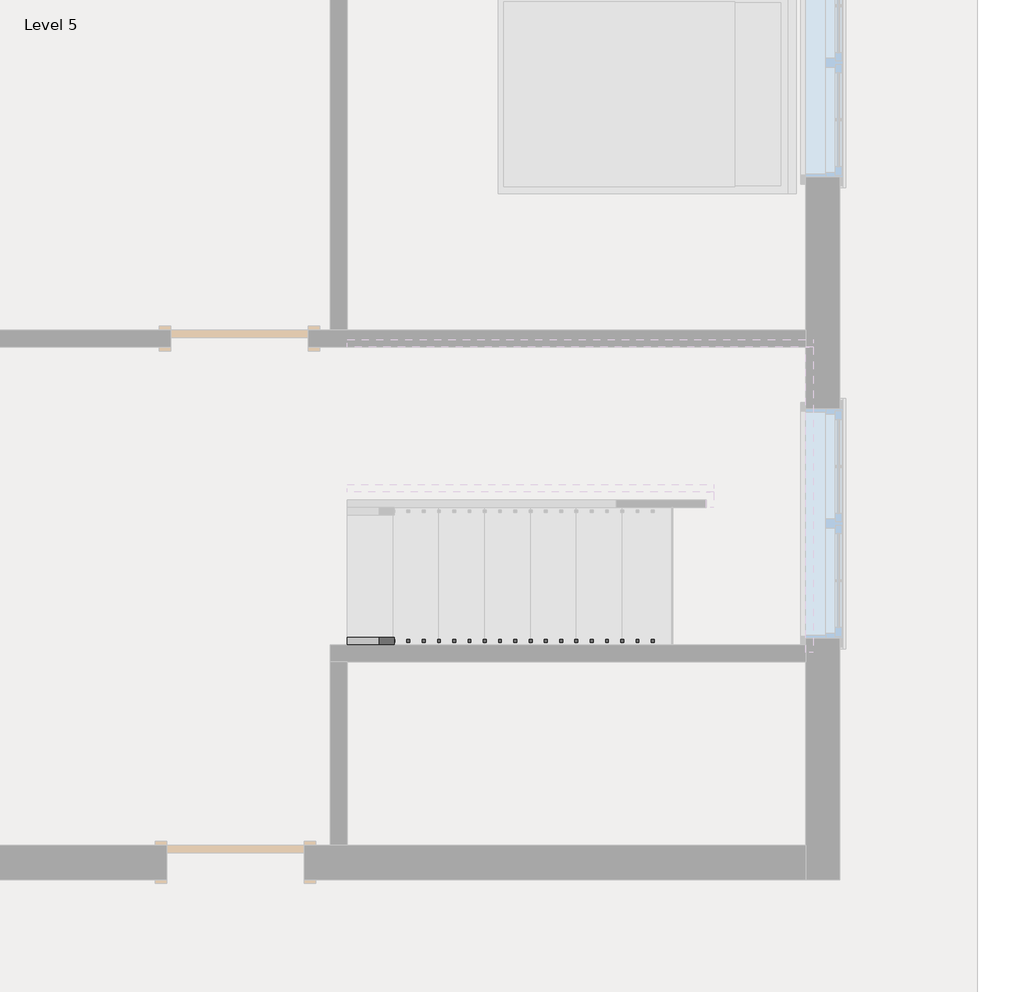
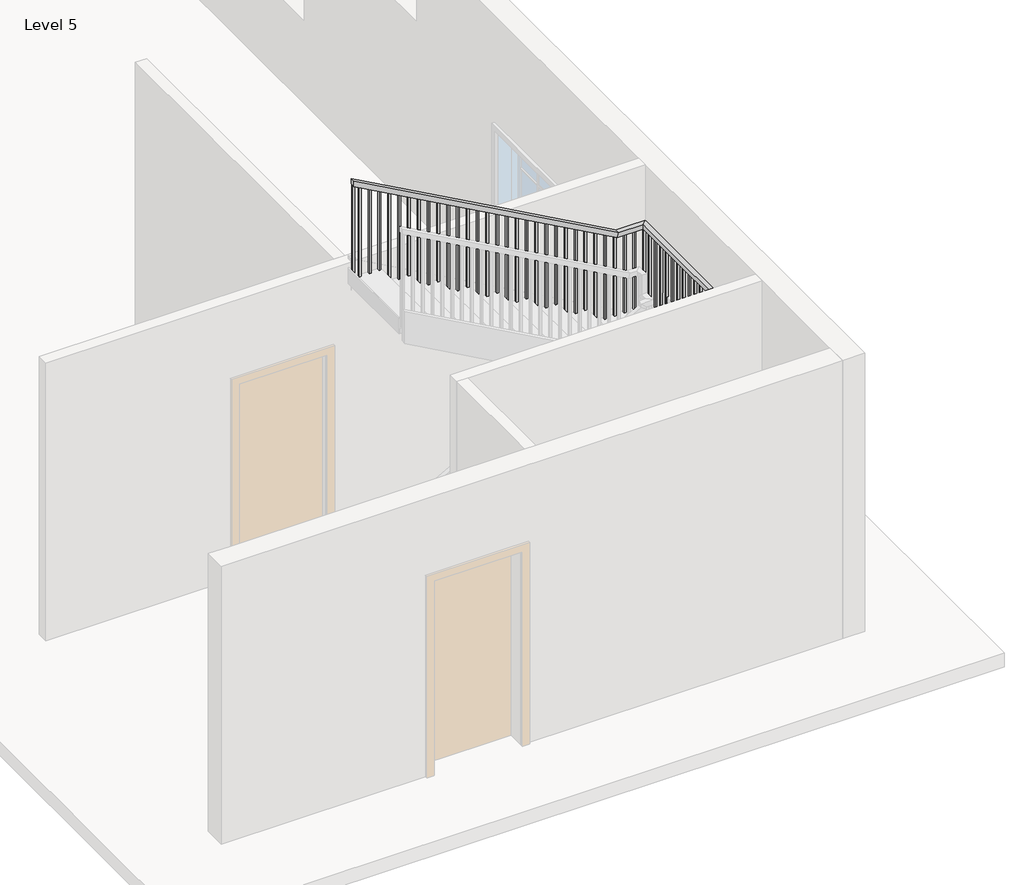
# One storey, part 2 of 3: 1 railing.
"""IFC4 building model written with IfcOpenShell, lengths in millimetres."""

from ifc_helpers import new_model, si_unit, frame, origin, place, context, project, spatial, polyline, outline, extrude, faceted_brep, element, save

model = new_model("IFC4")

# Units and contexts
model_context = context("Model", 3, world=origin())
ifc_project = project(units=[si_unit("LENGTHUNIT", "METRE", prefix="MILLI")], contexts=[model_context])

# Site, building, storey
site = spatial("IfcSite", under=ifc_project)
building = spatial("IfcBuilding", under=site)
storey = spatial("IfcBuildingStorey", under=building, Name="Level 5", Elevation=12649.2)

# Railing
placement = place(None, origin())
element("IfcRailing", 1, ObjectType="Handrail - Rectangular", at=placement, inside=storey, context=model_context, shape_type="SolidModel", body=[
    faceted_brep([(-1197.97188, -4765.70869, 13732.9333333), (-1197.97188, -4765.70869, 13674.820221), (-1197.97188, -4816.50869, 13674.820221), (-1197.97188, -4816.50869, 13732.9333333), (1240.42812, -4765.70869, 15087.6), (1253.5917222, -4765.70869, 15036.8), (1253.5917222, -4816.50869, 15036.8), (1240.42812, -4816.50869, 15087.6), (1799.22812, -4765.70869, 15087.6), (1799.22812, -4765.70869, 15036.8), (1850.02812, -4816.50869, 15036.8), (1850.02812, -4816.50869, 15087.6), (1799.22812, -2886.10869, 15087.6), (1799.22812, -2886.10869, 15036.8), (1850.02812, -2835.30869, 15036.8), (1850.02812, -2835.30869, 15087.6), (1545.22812, -2886.10869, 15087.6), (1532.0645177, -2886.10869, 15036.8), (1532.0645177, -2835.30869, 15036.8), (1545.22812, -2835.30869, 15087.6), (-1197.97188, -2886.10869, 16611.6), (-1197.97188, -2835.30869, 16611.6), (-1197.97188, -2835.30869, 16553.4868876), (-1197.97188, -2886.10869, 16553.4868876)], [[[0, 1, 2, 3]], [[1, 0, 4, 5]], [[2, 1, 5, 6]], [[3, 2, 6, 7]], [[0, 3, 7, 4]], [[5, 4, 8, 9]], [[6, 5, 9, 10]], [[7, 6, 10, 11]], [[4, 7, 11, 8]], [[9, 8, 12, 13]], [[10, 9, 13, 14]], [[11, 10, 14, 15]], [[8, 11, 15, 12]], [[13, 12, 16, 17]], [[14, 13, 17, 18]], [[15, 14, 18, 19]], [[12, 15, 19, 16]], [[20, 21, 22, 23]], [[17, 16, 20, 23]], [[18, 17, 23, 22]], [[19, 18, 22, 21]], [[16, 19, 21, 20]]]),
    extrude(outline(polyline([(16505.8618876, -1112.24688), (16516.445221, -1131.29688), (15527.8666667, -1131.29688), (15527.8666667, -1112.24688), (16505.8618876, -1112.24688)])), frame((0.0, -2870.23369, 0.0), z_axis=(0.0, 1.0, 0.0), x_axis=(0.0, 0.0, 1.0)), (0.0, 0.0, 1.0), 19.05),
    extrude(outline(polyline([(16449.4174432, -1010.64688), (16460.0007765, -1029.69688), (15527.8666667, -1029.69688), (15527.8666667, -1010.64688), (16449.4174432, -1010.64688)])), frame((0.0, -2870.23369, 0.0), z_axis=(0.0, 1.0, 0.0), x_axis=(0.0, 0.0, 1.0)), (0.0, 0.0, 1.0), 19.05),
    extrude(outline(polyline([(16392.9729988, -909.04688), (16403.5563321, -928.09688), (15527.8666667, -928.09688), (15527.8666667, -909.04688), (16392.9729988, -909.04688)])), frame((0.0, -2870.23369, 0.0), z_axis=(0.0, 1.0, 0.0), x_axis=(0.0, 0.0, 1.0)), (0.0, 0.0, 1.0), 19.05),
    extrude(outline(polyline([(16336.5285543, -807.44688), (16347.1118876, -826.49688), (15358.5333333, -826.49688), (15358.5333333, -807.44688), (16336.5285543, -807.44688)])), frame((0.0, -2870.23369, 0.0), z_axis=(0.0, 1.0, 0.0), x_axis=(0.0, 0.0, 1.0)), (0.0, 0.0, 1.0), 19.05),
    extrude(outline(polyline([(16280.0841099, -705.84688), (16290.6674432, -724.89688), (15358.5333333, -724.89688), (15358.5333333, -705.84688), (16280.0841099, -705.84688)])), frame((0.0, -2870.23369, 0.0), z_axis=(0.0, 1.0, 0.0), x_axis=(0.0, 0.0, 1.0)), (0.0, 0.0, 1.0), 19.05),
    extrude(outline(polyline([(16223.6396654, -604.24688), (16234.2229988, -623.29688), (15358.5333333, -623.29688), (15358.5333333, -604.24688), (16223.6396654, -604.24688)])), frame((0.0, -2870.23369, 0.0), z_axis=(0.0, 1.0, 0.0), x_axis=(0.0, 0.0, 1.0)), (0.0, 0.0, 1.0), 19.05),
    extrude(outline(polyline([(16167.195221, -502.64688), (16177.7785543, -521.69688), (15189.2, -521.69688), (15189.2, -502.64688), (16167.195221, -502.64688)])), frame((0.0, -2870.23369, 0.0), z_axis=(0.0, 1.0, 0.0), x_axis=(0.0, 0.0, 1.0)), (0.0, 0.0, 1.0), 19.05),
    extrude(outline(polyline([(16110.7507765, -401.04688), (16121.3341099, -420.09688), (15189.2, -420.09688), (15189.2, -401.04688), (16110.7507765, -401.04688)])), frame((0.0, -2870.23369, 0.0), z_axis=(0.0, 1.0, 0.0), x_axis=(0.0, 0.0, 1.0)), (0.0, 0.0, 1.0), 19.05),
    extrude(outline(polyline([(16054.3063321, -299.44688), (16064.8896654, -318.49688), (15189.2, -318.49688), (15189.2, -299.44688), (16054.3063321, -299.44688)])), frame((0.0, -2870.23369, 0.0), z_axis=(0.0, 1.0, 0.0), x_axis=(0.0, 0.0, 1.0)), (0.0, 0.0, 1.0), 19.05),
    extrude(outline(polyline([(15997.8618876, -197.84688), (16008.445221, -216.89688), (15019.8666667, -216.89688), (15019.8666667, -197.84688), (15997.8618876, -197.84688)])), frame((0.0, -2870.23369, 0.0), z_axis=(0.0, 1.0, 0.0), x_axis=(0.0, 0.0, 1.0)), (0.0, 0.0, 1.0), 19.05),
    extrude(outline(polyline([(15941.4174432, -96.24688), (15952.0007765, -115.29688), (15019.8666667, -115.29688), (15019.8666667, -96.24688), (15941.4174432, -96.24688)])), frame((0.0, -2870.23369, 0.0), z_axis=(0.0, 1.0, 0.0), x_axis=(0.0, 0.0, 1.0)), (0.0, 0.0, 1.0), 19.05),
    extrude(outline(polyline([(15884.9729988, 5.35312), (15895.5563321, -13.69688), (15019.8666667, -13.69688), (15019.8666667, 5.35312), (15884.9729988, 5.35312)])), frame((0.0, -2870.23369, 0.0), z_axis=(0.0, 1.0, 0.0), x_axis=(0.0, 0.0, 1.0)), (0.0, 0.0, 1.0), 19.05),
    extrude(outline(polyline([(15828.5285543, 106.95312), (15839.1118876, 87.90312), (14850.5333333, 87.90312), (14850.5333333, 106.95312), (15828.5285543, 106.95312)])), frame((0.0, -2870.23369, 0.0), z_axis=(0.0, 1.0, 0.0), x_axis=(0.0, 0.0, 1.0)), (0.0, 0.0, 1.0), 19.05),
    extrude(outline(polyline([(15772.0841099, 208.55312), (15782.6674432, 189.50312), (14850.5333333, 189.50312), (14850.5333333, 208.55312), (15772.0841099, 208.55312)])), frame((0.0, -2870.23369, 0.0), z_axis=(0.0, 1.0, 0.0), x_axis=(0.0, 0.0, 1.0)), (0.0, 0.0, 1.0), 19.05),
    extrude(outline(polyline([(15715.6396654, 310.15312), (15726.2229988, 291.10312), (14850.5333333, 291.10312), (14850.5333333, 310.15312), (15715.6396654, 310.15312)])), frame((0.0, -2870.23369, 0.0), z_axis=(0.0, 1.0, 0.0), x_axis=(0.0, 0.0, 1.0)), (0.0, 0.0, 1.0), 19.05),
    extrude(outline(polyline([(15659.195221, 411.75312), (15669.7785543, 392.70312), (14681.2, 392.70312), (14681.2, 411.75312), (15659.195221, 411.75312)])), frame((0.0, -2870.23369, 0.0), z_axis=(0.0, 1.0, 0.0), x_axis=(0.0, 0.0, 1.0)), (0.0, 0.0, 1.0), 19.05),
    extrude(outline(polyline([(15602.7507765, 513.35312), (15613.3341099, 494.30312), (14681.2, 494.30312), (14681.2, 513.35312), (15602.7507765, 513.35312)])), frame((0.0, -2870.23369, 0.0), z_axis=(0.0, 1.0, 0.0), x_axis=(0.0, 0.0, 1.0)), (0.0, 0.0, 1.0), 19.05),
    extrude(outline(polyline([(15546.3063321, 614.95312), (15556.8896654, 595.90312), (14681.2, 595.90312), (14681.2, 614.95312), (15546.3063321, 614.95312)])), frame((0.0, -2870.23369, 0.0), z_axis=(0.0, 1.0, 0.0), x_axis=(0.0, 0.0, 1.0)), (0.0, 0.0, 1.0), 19.05),
    extrude(outline(polyline([(15489.8618876, 716.55312), (15500.445221, 697.50312), (14511.8666667, 697.50312), (14511.8666667, 716.55312), (15489.8618876, 716.55312)])), frame((0.0, -2870.23369, 0.0), z_axis=(0.0, 1.0, 0.0), x_axis=(0.0, 0.0, 1.0)), (0.0, 0.0, 1.0), 19.05),
    extrude(outline(polyline([(15433.4174432, 818.15312), (15444.0007765, 799.10312), (14511.8666667, 799.10312), (14511.8666667, 818.15312), (15433.4174432, 818.15312)])), frame((0.0, -2870.23369, 0.0), z_axis=(0.0, 1.0, 0.0), x_axis=(0.0, 0.0, 1.0)), (0.0, 0.0, 1.0), 19.05),
    extrude(outline(polyline([(15376.9729988, 919.75312), (15387.5563321, 900.70312), (14511.8666667, 900.70312), (14511.8666667, 919.75312), (15376.9729988, 919.75312)])), frame((0.0, -2870.23369, 0.0), z_axis=(0.0, 1.0, 0.0), x_axis=(0.0, 0.0, 1.0)), (0.0, 0.0, 1.0), 19.05),
    extrude(outline(polyline([(15320.5285543, 1021.35312), (15331.1118876, 1002.30312), (14342.5333333, 1002.30312), (14342.5333333, 1021.35312), (15320.5285543, 1021.35312)])), frame((0.0, -2870.23369, 0.0), z_axis=(0.0, 1.0, 0.0), x_axis=(0.0, 0.0, 1.0)), (0.0, 0.0, 1.0), 19.05),
    extrude(outline(polyline([(15264.0841099, 1122.95312), (15274.6674432, 1103.90312), (14342.5333333, 1103.90312), (14342.5333333, 1122.95312), (15264.0841099, 1122.95312)])), frame((0.0, -2870.23369, 0.0), z_axis=(0.0, 1.0, 0.0), x_axis=(0.0, 0.0, 1.0)), (0.0, 0.0, 1.0), 19.05),
    extrude(outline(polyline([(15207.6396654, 1224.55312), (15218.2229988, 1205.50312), (14342.5333333, 1205.50312), (14342.5333333, 1224.55312), (15207.6396654, 1224.55312)])), frame((0.0, -2870.23369, 0.0), z_axis=(0.0, 1.0, 0.0), x_axis=(0.0, 0.0, 1.0)), (0.0, 0.0, 1.0), 19.05),
    extrude(outline(polyline([(15151.195221, 1326.15312), (15161.7785543, 1307.10312), (14173.2, 1307.10312), (14173.2, 1326.15312), (15151.195221, 1326.15312)])), frame((0.0, -2870.23369, 0.0), z_axis=(0.0, 1.0, 0.0), x_axis=(0.0, 0.0, 1.0)), (0.0, 0.0, 1.0), 19.05),
    extrude(outline(polyline([(15094.7507765, 1427.75312), (15105.3341099, 1408.70312), (14173.2, 1408.70312), (14173.2, 1427.75312), (15094.7507765, 1427.75312)])), frame((0.0, -2870.23369, 0.0), z_axis=(0.0, 1.0, 0.0), x_axis=(0.0, 0.0, 1.0)), (0.0, 0.0, 1.0), 19.05),
    extrude(outline(polyline([(15038.3063321, 1529.35312), (15048.8896654, 1510.30312), (14173.2, 1510.30312), (14173.2, 1529.35312), (15038.3063321, 1529.35312)])), frame((0.0, -2870.23369, 0.0), z_axis=(0.0, 1.0, 0.0), x_axis=(0.0, 0.0, 1.0)), (0.0, 0.0, 1.0), 19.05),
    extrude(outline(polyline([(1630.95312, -2851.18369), (1630.95312, -2870.23369), (1611.90312, -2870.23369), (1611.90312, -2851.18369), (1630.95312, -2851.18369)])), frame((0.0, 0.0, 14173.2), z_axis=(0.0, 0.0, 1.0), x_axis=(1.0, 0.0, 0.0)), (0.0, 0.0, 1.0), 863.6),
    extrude(outline(polyline([(1732.55312, -2851.18369), (1732.55312, -2870.23369), (1713.50312, -2870.23369), (1713.50312, -2851.18369), (1732.55312, -2851.18369)])), frame((0.0, 0.0, 14173.2), z_axis=(0.0, 0.0, 1.0), x_axis=(1.0, 0.0, 0.0)), (0.0, 0.0, 1.0), 863.6),
    extrude(outline(polyline([(1834.15312, -2971.83369), (1815.10312, -2971.83369), (1815.10312, -2952.78369), (1834.15312, -2952.78369), (1834.15312, -2971.83369)])), frame((0.0, 0.0, 14173.2), z_axis=(0.0, 0.0, 1.0), x_axis=(1.0, 0.0, 0.0)), (0.0, 0.0, 1.0), 863.6),
    extrude(outline(polyline([(1834.15312, -3073.43369), (1815.10312, -3073.43369), (1815.10312, -3054.38369), (1834.15312, -3054.38369), (1834.15312, -3073.43369)])), frame((0.0, 0.0, 14173.2), z_axis=(0.0, 0.0, 1.0), x_axis=(1.0, 0.0, 0.0)), (0.0, 0.0, 1.0), 863.6),
    extrude(outline(polyline([(1834.15312, -3175.03369), (1815.10312, -3175.03369), (1815.10312, -3155.98369), (1834.15312, -3155.98369), (1834.15312, -3175.03369)])), frame((0.0, 0.0, 14173.2), z_axis=(0.0, 0.0, 1.0), x_axis=(1.0, 0.0, 0.0)), (0.0, 0.0, 1.0), 863.6),
    extrude(outline(polyline([(1834.15312, -3276.63369), (1815.10312, -3276.63369), (1815.10312, -3257.58369), (1834.15312, -3257.58369), (1834.15312, -3276.63369)])), frame((0.0, 0.0, 14173.2), z_axis=(0.0, 0.0, 1.0), x_axis=(1.0, 0.0, 0.0)), (0.0, 0.0, 1.0), 863.6),
    extrude(outline(polyline([(1834.15312, -3378.23369), (1815.10312, -3378.23369), (1815.10312, -3359.18369), (1834.15312, -3359.18369), (1834.15312, -3378.23369)])), frame((0.0, 0.0, 14173.2), z_axis=(0.0, 0.0, 1.0), x_axis=(1.0, 0.0, 0.0)), (0.0, 0.0, 1.0), 863.6),
    extrude(outline(polyline([(1834.15312, -3479.83369), (1815.10312, -3479.83369), (1815.10312, -3460.78369), (1834.15312, -3460.78369), (1834.15312, -3479.83369)])), frame((0.0, 0.0, 14173.2), z_axis=(0.0, 0.0, 1.0), x_axis=(1.0, 0.0, 0.0)), (0.0, 0.0, 1.0), 863.6),
    extrude(outline(polyline([(1834.15312, -3581.43369), (1815.10312, -3581.43369), (1815.10312, -3562.38369), (1834.15312, -3562.38369), (1834.15312, -3581.43369)])), frame((0.0, 0.0, 14173.2), z_axis=(0.0, 0.0, 1.0), x_axis=(1.0, 0.0, 0.0)), (0.0, 0.0, 1.0), 863.6),
    extrude(outline(polyline([(1834.15312, -3683.03369), (1815.10312, -3683.03369), (1815.10312, -3663.98369), (1834.15312, -3663.98369), (1834.15312, -3683.03369)])), frame((0.0, 0.0, 14173.2), z_axis=(0.0, 0.0, 1.0), x_axis=(1.0, 0.0, 0.0)), (0.0, 0.0, 1.0), 863.6),
    extrude(outline(polyline([(1834.15312, -3784.63369), (1815.10312, -3784.63369), (1815.10312, -3765.58369), (1834.15312, -3765.58369), (1834.15312, -3784.63369)])), frame((0.0, 0.0, 14173.2), z_axis=(0.0, 0.0, 1.0), x_axis=(1.0, 0.0, 0.0)), (0.0, 0.0, 1.0), 863.6),
    extrude(outline(polyline([(1834.15312, -3886.23369), (1815.10312, -3886.23369), (1815.10312, -3867.18369), (1834.15312, -3867.18369), (1834.15312, -3886.23369)])), frame((0.0, 0.0, 14173.2), z_axis=(0.0, 0.0, 1.0), x_axis=(1.0, 0.0, 0.0)), (0.0, 0.0, 1.0), 863.6),
    extrude(outline(polyline([(1834.15312, -3987.83369), (1815.10312, -3987.83369), (1815.10312, -3968.78369), (1834.15312, -3968.78369), (1834.15312, -3987.83369)])), frame((0.0, 0.0, 14173.2), z_axis=(0.0, 0.0, 1.0), x_axis=(1.0, 0.0, 0.0)), (0.0, 0.0, 1.0), 863.6),
    extrude(outline(polyline([(1834.15312, -4089.43369), (1815.10312, -4089.43369), (1815.10312, -4070.38369), (1834.15312, -4070.38369), (1834.15312, -4089.43369)])), frame((0.0, 0.0, 14173.2), z_axis=(0.0, 0.0, 1.0), x_axis=(1.0, 0.0, 0.0)), (0.0, 0.0, 1.0), 863.6),
    extrude(outline(polyline([(1834.15312, -4191.03369), (1815.10312, -4191.03369), (1815.10312, -4171.98369), (1834.15312, -4171.98369), (1834.15312, -4191.03369)])), frame((0.0, 0.0, 14173.2), z_axis=(0.0, 0.0, 1.0), x_axis=(1.0, 0.0, 0.0)), (0.0, 0.0, 1.0), 863.6),
    extrude(outline(polyline([(1834.15312, -4292.63369), (1815.10312, -4292.63369), (1815.10312, -4273.58369), (1834.15312, -4273.58369), (1834.15312, -4292.63369)])), frame((0.0, 0.0, 14173.2), z_axis=(0.0, 0.0, 1.0), x_axis=(1.0, 0.0, 0.0)), (0.0, 0.0, 1.0), 863.6),
    extrude(outline(polyline([(1834.15312, -4394.23369), (1815.10312, -4394.23369), (1815.10312, -4375.18369), (1834.15312, -4375.18369), (1834.15312, -4394.23369)])), frame((0.0, 0.0, 14173.2), z_axis=(0.0, 0.0, 1.0), x_axis=(1.0, 0.0, 0.0)), (0.0, 0.0, 1.0), 863.6),
    extrude(outline(polyline([(1834.15312, -4495.83369), (1815.10312, -4495.83369), (1815.10312, -4476.78369), (1834.15312, -4476.78369), (1834.15312, -4495.83369)])), frame((0.0, 0.0, 14173.2), z_axis=(0.0, 0.0, 1.0), x_axis=(1.0, 0.0, 0.0)), (0.0, 0.0, 1.0), 863.6),
    extrude(outline(polyline([(1834.15312, -4597.43369), (1815.10312, -4597.43369), (1815.10312, -4578.38369), (1834.15312, -4578.38369), (1834.15312, -4597.43369)])), frame((0.0, 0.0, 14173.2), z_axis=(0.0, 0.0, 1.0), x_axis=(1.0, 0.0, 0.0)), (0.0, 0.0, 1.0), 863.6),
    extrude(outline(polyline([(1834.15312, -4699.03369), (1815.10312, -4699.03369), (1815.10312, -4679.98369), (1834.15312, -4679.98369), (1834.15312, -4699.03369)])), frame((0.0, 0.0, 14173.2), z_axis=(0.0, 0.0, 1.0), x_axis=(1.0, 0.0, 0.0)), (0.0, 0.0, 1.0), 863.6),
    extrude(outline(polyline([(1738.90312, -4800.63369), (1738.90312, -4781.58369), (1757.95312, -4781.58369), (1757.95312, -4800.63369), (1738.90312, -4800.63369)])), frame((0.0, 0.0, 14173.2), z_axis=(0.0, 0.0, 1.0), x_axis=(1.0, 0.0, 0.0)), (0.0, 0.0, 1.0), 863.6),
    extrude(outline(polyline([(1637.30312, -4800.63369), (1637.30312, -4781.58369), (1656.35312, -4781.58369), (1656.35312, -4800.63369), (1637.30312, -4800.63369)])), frame((0.0, 0.0, 14173.2), z_axis=(0.0, 0.0, 1.0), x_axis=(1.0, 0.0, 0.0)), (0.0, 0.0, 1.0), 863.6),
    extrude(outline(polyline([(1535.70312, -4800.63369), (1535.70312, -4781.58369), (1554.75312, -4781.58369), (1554.75312, -4800.63369), (1535.70312, -4800.63369)])), frame((0.0, 0.0, 14173.2), z_axis=(0.0, 0.0, 1.0), x_axis=(1.0, 0.0, 0.0)), (0.0, 0.0, 1.0), 863.6),
    extrude(outline(polyline([(1434.10312, -4800.63369), (1434.10312, -4781.58369), (1453.15312, -4781.58369), (1453.15312, -4800.63369), (1434.10312, -4800.63369)])), frame((0.0, 0.0, 14173.2), z_axis=(0.0, 0.0, 1.0), x_axis=(1.0, 0.0, 0.0)), (0.0, 0.0, 1.0), 863.6),
    extrude(outline(polyline([(1332.50312, -4800.63369), (1332.50312, -4781.58369), (1351.55312, -4781.58369), (1351.55312, -4800.63369), (1332.50312, -4800.63369)])), frame((0.0, 0.0, 14173.2), z_axis=(0.0, 0.0, 1.0), x_axis=(1.0, 0.0, 0.0)), (0.0, 0.0, 1.0), 863.6),
    extrude(outline(polyline([(15034.7785543, 1249.95312), (15024.195221, 1230.90312), (14173.2, 1230.90312), (14173.2, 1249.95312), (15034.7785543, 1249.95312)])), frame((0.0, -4800.63369, 0.0), z_axis=(0.0, 1.0, 0.0), x_axis=(0.0, 0.0, 1.0)), (0.0, 0.0, 1.0), 19.05),
    extrude(outline(polyline([(14978.3341099, 1148.35312), (14967.7507765, 1129.30312), (14003.8666667, 1129.30312), (14003.8666667, 1148.35312), (14978.3341099, 1148.35312)])), frame((0.0, -4800.63369, 0.0), z_axis=(0.0, 1.0, 0.0), x_axis=(0.0, 0.0, 1.0)), (0.0, 0.0, 1.0), 19.05),
    extrude(outline(polyline([(14921.8896654, 1046.75312), (14911.3063321, 1027.70312), (14003.8666667, 1027.70312), (14003.8666667, 1046.75312), (14921.8896654, 1046.75312)])), frame((0.0, -4800.63369, 0.0), z_axis=(0.0, 1.0, 0.0), x_axis=(0.0, 0.0, 1.0)), (0.0, 0.0, 1.0), 19.05),
    extrude(outline(polyline([(14865.445221, 945.15312), (14854.8618876, 926.10312), (14003.8666667, 926.10312), (14003.8666667, 945.15312), (14865.445221, 945.15312)])), frame((0.0, -4800.63369, 0.0), z_axis=(0.0, 1.0, 0.0), x_axis=(0.0, 0.0, 1.0)), (0.0, 0.0, 1.0), 19.05),
    extrude(outline(polyline([(14809.0007765, 843.55312), (14798.4174432, 824.50312), (13834.5333333, 824.50312), (13834.5333333, 843.55312), (14809.0007765, 843.55312)])), frame((0.0, -4800.63369, 0.0), z_axis=(0.0, 1.0, 0.0), x_axis=(0.0, 0.0, 1.0)), (0.0, 0.0, 1.0), 19.05),
    extrude(outline(polyline([(14752.5563321, 741.95312), (14741.9729988, 722.90312), (13834.5333333, 722.90312), (13834.5333333, 741.95312), (14752.5563321, 741.95312)])), frame((0.0, -4800.63369, 0.0), z_axis=(0.0, 1.0, 0.0), x_axis=(0.0, 0.0, 1.0)), (0.0, 0.0, 1.0), 19.05),
    extrude(outline(polyline([(14696.1118876, 640.35312), (14685.5285543, 621.30312), (13834.5333333, 621.30312), (13834.5333333, 640.35312), (14696.1118876, 640.35312)])), frame((0.0, -4800.63369, 0.0), z_axis=(0.0, 1.0, 0.0), x_axis=(0.0, 0.0, 1.0)), (0.0, 0.0, 1.0), 19.05),
    extrude(outline(polyline([(14639.6674432, 538.75312), (14629.0841099, 519.70312), (13665.2, 519.70312), (13665.2, 538.75312), (14639.6674432, 538.75312)])), frame((0.0, -4800.63369, 0.0), z_axis=(0.0, 1.0, 0.0), x_axis=(0.0, 0.0, 1.0)), (0.0, 0.0, 1.0), 19.05),
    extrude(outline(polyline([(14583.2229988, 437.15312), (14572.6396654, 418.10312), (13665.2, 418.10312), (13665.2, 437.15312), (14583.2229988, 437.15312)])), frame((0.0, -4800.63369, 0.0), z_axis=(0.0, 1.0, 0.0), x_axis=(0.0, 0.0, 1.0)), (0.0, 0.0, 1.0), 19.05),
    extrude(outline(polyline([(14526.7785543, 335.55312), (14516.195221, 316.50312), (13665.2, 316.50312), (13665.2, 335.55312), (14526.7785543, 335.55312)])), frame((0.0, -4800.63369, 0.0), z_axis=(0.0, 1.0, 0.0), x_axis=(0.0, 0.0, 1.0)), (0.0, 0.0, 1.0), 19.05),
    extrude(outline(polyline([(14470.3341099, 233.95312), (14459.7507765, 214.90312), (13495.8666667, 214.90312), (13495.8666667, 233.95312), (14470.3341099, 233.95312)])), frame((0.0, -4800.63369, 0.0), z_axis=(0.0, 1.0, 0.0), x_axis=(0.0, 0.0, 1.0)), (0.0, 0.0, 1.0), 19.05),
    extrude(outline(polyline([(14413.8896654, 132.35312), (14403.3063321, 113.30312), (13495.8666667, 113.30312), (13495.8666667, 132.35312), (14413.8896654, 132.35312)])), frame((0.0, -4800.63369, 0.0), z_axis=(0.0, 1.0, 0.0), x_axis=(0.0, 0.0, 1.0)), (0.0, 0.0, 1.0), 19.05),
    extrude(outline(polyline([(14357.445221, 30.75312), (14346.8618876, 11.70312), (13495.8666667, 11.70312), (13495.8666667, 30.75312), (14357.445221, 30.75312)])), frame((0.0, -4800.63369, 0.0), z_axis=(0.0, 1.0, 0.0), x_axis=(0.0, 0.0, 1.0)), (0.0, 0.0, 1.0), 19.05),
    extrude(outline(polyline([(14301.0007765, -70.84688), (14290.4174432, -89.89688), (13326.5333333, -89.89688), (13326.5333333, -70.84688), (14301.0007765, -70.84688)])), frame((0.0, -4800.63369, 0.0), z_axis=(0.0, 1.0, 0.0), x_axis=(0.0, 0.0, 1.0)), (0.0, 0.0, 1.0), 19.05),
    extrude(outline(polyline([(14244.5563321, -172.44688), (14233.9729988, -191.49688), (13326.5333333, -191.49688), (13326.5333333, -172.44688), (14244.5563321, -172.44688)])), frame((0.0, -4800.63369, 0.0), z_axis=(0.0, 1.0, 0.0), x_axis=(0.0, 0.0, 1.0)), (0.0, 0.0, 1.0), 19.05),
    extrude(outline(polyline([(14188.1118876, -274.04688), (14177.5285543, -293.09688), (13326.5333333, -293.09688), (13326.5333333, -274.04688), (14188.1118876, -274.04688)])), frame((0.0, -4800.63369, 0.0), z_axis=(0.0, 1.0, 0.0), x_axis=(0.0, 0.0, 1.0)), (0.0, 0.0, 1.0), 19.05),
    extrude(outline(polyline([(14131.6674432, -375.64688), (14121.0841099, -394.69688), (13157.2, -394.69688), (13157.2, -375.64688), (14131.6674432, -375.64688)])), frame((0.0, -4800.63369, 0.0), z_axis=(0.0, 1.0, 0.0), x_axis=(0.0, 0.0, 1.0)), (0.0, 0.0, 1.0), 19.05),
    extrude(outline(polyline([(14075.2229988, -477.24688), (14064.6396654, -496.29688), (13157.2, -496.29688), (13157.2, -477.24688), (14075.2229988, -477.24688)])), frame((0.0, -4800.63369, 0.0), z_axis=(0.0, 1.0, 0.0), x_axis=(0.0, 0.0, 1.0)), (0.0, 0.0, 1.0), 19.05),
    extrude(outline(polyline([(14018.7785543, -578.84688), (14008.195221, -597.89688), (13157.2, -597.89688), (13157.2, -578.84688), (14018.7785543, -578.84688)])), frame((0.0, -4800.63369, 0.0), z_axis=(0.0, 1.0, 0.0), x_axis=(0.0, 0.0, 1.0)), (0.0, 0.0, 1.0), 19.05),
    extrude(outline(polyline([(13962.3341099, -680.44688), (13951.7507765, -699.49688), (12987.8666667, -699.49688), (12987.8666667, -680.44688), (13962.3341099, -680.44688)])), frame((0.0, -4800.63369, 0.0), z_axis=(0.0, 1.0, 0.0), x_axis=(0.0, 0.0, 1.0)), (0.0, 0.0, 1.0), 19.05),
    extrude(outline(polyline([(13905.8896654, -782.04688), (13895.3063321, -801.09688), (12987.8666667, -801.09688), (12987.8666667, -782.04688), (13905.8896654, -782.04688)])), frame((0.0, -4800.63369, 0.0), z_axis=(0.0, 1.0, 0.0), x_axis=(0.0, 0.0, 1.0)), (0.0, 0.0, 1.0), 19.05),
    extrude(outline(polyline([(13849.445221, -883.64688), (13838.8618876, -902.69688), (12987.8666667, -902.69688), (12987.8666667, -883.64688), (13849.445221, -883.64688)])), frame((0.0, -4800.63369, 0.0), z_axis=(0.0, 1.0, 0.0), x_axis=(0.0, 0.0, 1.0)), (0.0, 0.0, 1.0), 19.05),
    extrude(outline(polyline([(13793.0007765, -985.24688), (13782.4174432, -1004.29688), (12818.5333333, -1004.29688), (12818.5333333, -985.24688), (13793.0007765, -985.24688)])), frame((0.0, -4800.63369, 0.0), z_axis=(0.0, 1.0, 0.0), x_axis=(0.0, 0.0, 1.0)), (0.0, 0.0, 1.0), 19.05),
    extrude(outline(polyline([(13736.5563321, -1086.84688), (13725.9729988, -1105.89688), (12818.5333333, -1105.89688), (12818.5333333, -1086.84688), (13736.5563321, -1086.84688)])), frame((0.0, -4800.63369, 0.0), z_axis=(0.0, 1.0, 0.0), x_axis=(0.0, 0.0, 1.0)), (0.0, 0.0, 1.0), 19.05),
    extrude(outline(polyline([(1834.15312, -2870.23369), (1815.10312, -2870.23369), (1815.10312, -2851.18369), (1834.15312, -2851.18369), (1834.15312, -2870.23369)])), frame((0.0, 0.0, 14173.2), z_axis=(0.0, 0.0, 1.0), x_axis=(1.0, 0.0, 0.0)), (0.0, 0.0, 1.0), 863.6),
    extrude(outline(polyline([(1815.10312, -4800.63369), (1815.10312, -4781.58369), (1834.15312, -4781.58369), (1834.15312, -4800.63369), (1815.10312, -4800.63369)])), frame((0.0, 0.0, 14173.2), z_axis=(0.0, 0.0, 1.0), x_axis=(1.0, 0.0, 0.0)), (0.0, 0.0, 1.0), 863.6),
    extrude(outline(polyline([(16542.9035543, -1178.92188), (16553.4868876, -1197.97188), (15527.8666667, -1197.97188), (15527.8666667, -1178.92188), (16542.9035543, -1178.92188)])), frame((0.0, -2870.23369, 0.0), z_axis=(0.0, 1.0, 0.0), x_axis=(0.0, 0.0, 1.0)), (0.0, 0.0, 1.0), 19.05),
    extrude(outline(polyline([(13685.4035543, -1178.92188), (13674.820221, -1197.97188), (12818.5333333, -1197.97188), (12818.5333333, -1178.92188), (13685.4035543, -1178.92188)])), frame((0.0, -4800.63369, 0.0), z_axis=(0.0, 1.0, 0.0), x_axis=(0.0, 0.0, 1.0)), (0.0, 0.0, 1.0), 19.05),
])

save(model, "model.ifc")

# Revit data of these elements
# Type "Handrail - Rectangular"
#   Assembly Code = "C2010400"
#   built-in parameter 1008612 = 0.0416667 (stored number, unit not read)
#   built-in parameter 1008611 = 0.0416667 (stored number, unit not read)
#   built-in parameter 1008609 = 0.333333 (stored number, unit not read)
#   built-in parameter 1008604 = 0.166667 (stored number, unit not read)
#   built-in parameter 1008603 = 0.166667 (stored number, unit not read)
#   Railing Height = 3' - 0"
#   built-in parameter 1008630 = 2
#   built-in parameter 1008610 = 2
#   built-in parameter 1008618 = Baluster - Square : 3/4"
# Element 1 (IfcRailing, "Handrail - Rectangular")
#   Phase Created = New Construction
